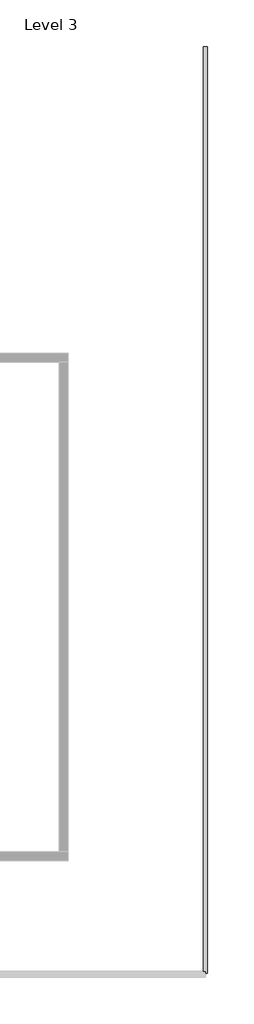
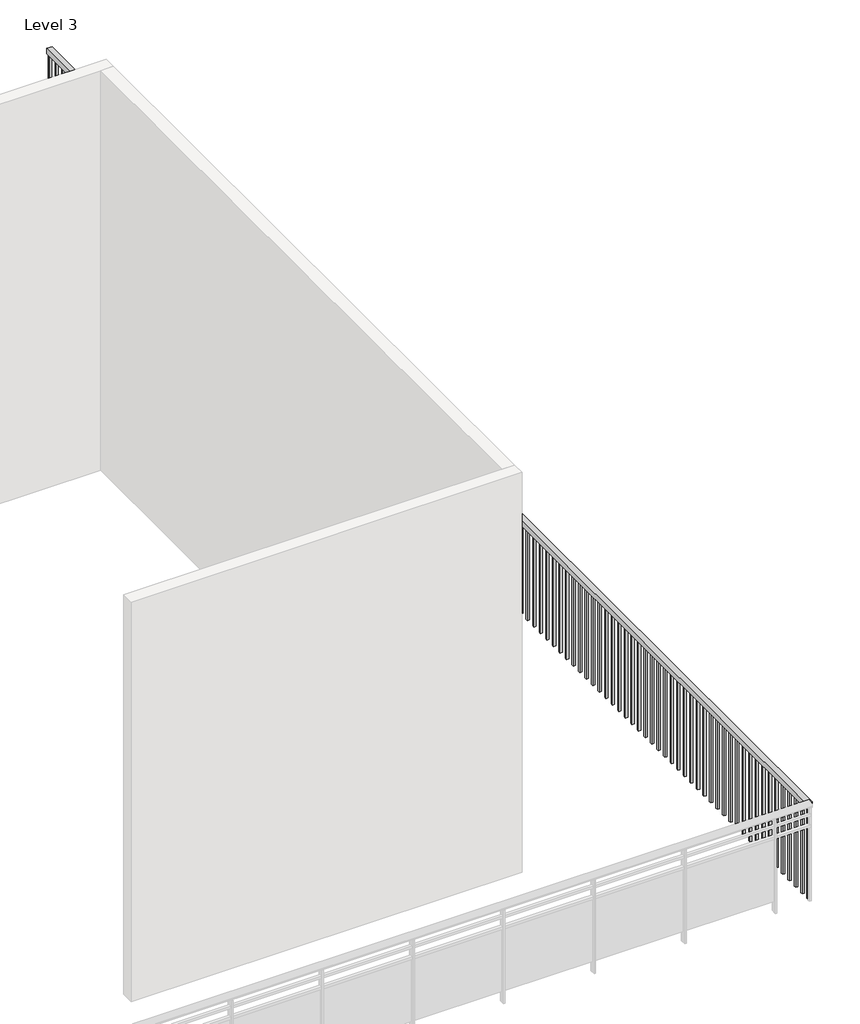
# One storey, part 2 of 2: 1 railing.
"""IFC4 building model written with IfcOpenShell, lengths in millimetres."""

from ifc_helpers import new_model, si_unit, frame, origin, place, context, project, spatial, polyline, outline, extrude, element, save

model = new_model("IFC4")

# Units and contexts
model_context = context("Model", 3, world=origin())
ifc_project = project(units=[si_unit("LENGTHUNIT", "METRE", prefix="MILLI")], contexts=[model_context])

# Site, building, storey
site = spatial("IfcSite", under=ifc_project)
building = spatial("IfcBuilding", under=site)
storey = spatial("IfcBuildingStorey", under=building, Name="Level 3", Elevation=3810.0)

# Railing
placement = place(None, origin())
element("IfcRailing", 1, ObjectType="Handrail - Rectangular", at=placement, inside=storey, context=model_context, shape_type="SweptSolid", body=[
    extrude(outline(polyline([(5557.6756121, -3130.6883122), (5506.8756121, -3130.6883122), (5506.8756121, 8667.6116878), (5557.6756121, 8667.6116878), (5557.6756121, -3130.6883122)])), frame((0.0, 0.0, 4673.6), z_axis=(0.0, 0.0, 1.0), x_axis=(1.0, 0.0, 0.0)), (0.0, 0.0, 1.0), 50.8),
    extrude(outline(polyline([(5541.8006121, 8645.3866878), (5522.7506121, 8645.3866878), (5522.7506121, 8664.4366878), (5541.8006121, 8664.4366878), (5541.8006121, 8645.3866878)])), frame((0.0, 0.0, 3810.0), z_axis=(0.0, 0.0, 1.0), x_axis=(1.0, 0.0, 0.0)), (0.0, 0.0, 1.0), 863.6),
    extrude(outline(polyline([(5541.8006121, 8543.7866878), (5522.7506121, 8543.7866878), (5522.7506121, 8562.8366878), (5541.8006121, 8562.8366878), (5541.8006121, 8543.7866878)])), frame((0.0, 0.0, 3810.0), z_axis=(0.0, 0.0, 1.0), x_axis=(1.0, 0.0, 0.0)), (0.0, 0.0, 1.0), 863.6),
    extrude(outline(polyline([(5541.8006121, 8442.1866878), (5522.7506121, 8442.1866878), (5522.7506121, 8461.2366878), (5541.8006121, 8461.2366878), (5541.8006121, 8442.1866878)])), frame((0.0, 0.0, 3810.0), z_axis=(0.0, 0.0, 1.0), x_axis=(1.0, 0.0, 0.0)), (0.0, 0.0, 1.0), 863.6),
    extrude(outline(polyline([(5541.8006121, 8340.5866878), (5522.7506121, 8340.5866878), (5522.7506121, 8359.6366878), (5541.8006121, 8359.6366878), (5541.8006121, 8340.5866878)])), frame((0.0, 0.0, 3810.0), z_axis=(0.0, 0.0, 1.0), x_axis=(1.0, 0.0, 0.0)), (0.0, 0.0, 1.0), 863.6),
    extrude(outline(polyline([(5541.8006121, 8238.9866878), (5522.7506121, 8238.9866878), (5522.7506121, 8258.0366878), (5541.8006121, 8258.0366878), (5541.8006121, 8238.9866878)])), frame((0.0, 0.0, 3810.0), z_axis=(0.0, 0.0, 1.0), x_axis=(1.0, 0.0, 0.0)), (0.0, 0.0, 1.0), 863.6),
    extrude(outline(polyline([(5541.8006121, 8137.3866878), (5522.7506121, 8137.3866878), (5522.7506121, 8156.4366878), (5541.8006121, 8156.4366878), (5541.8006121, 8137.3866878)])), frame((0.0, 0.0, 3810.0), z_axis=(0.0, 0.0, 1.0), x_axis=(1.0, 0.0, 0.0)), (0.0, 0.0, 1.0), 863.6),
    extrude(outline(polyline([(5541.8006121, 8035.7866878), (5522.7506121, 8035.7866878), (5522.7506121, 8054.8366878), (5541.8006121, 8054.8366878), (5541.8006121, 8035.7866878)])), frame((0.0, 0.0, 3810.0), z_axis=(0.0, 0.0, 1.0), x_axis=(1.0, 0.0, 0.0)), (0.0, 0.0, 1.0), 863.6),
    extrude(outline(polyline([(5541.8006121, 7934.1866878), (5522.7506121, 7934.1866878), (5522.7506121, 7953.2366878), (5541.8006121, 7953.2366878), (5541.8006121, 7934.1866878)])), frame((0.0, 0.0, 3810.0), z_axis=(0.0, 0.0, 1.0), x_axis=(1.0, 0.0, 0.0)), (0.0, 0.0, 1.0), 863.6),
    extrude(outline(polyline([(5541.8006121, 7832.5866878), (5522.7506121, 7832.5866878), (5522.7506121, 7851.6366878), (5541.8006121, 7851.6366878), (5541.8006121, 7832.5866878)])), frame((0.0, 0.0, 3810.0), z_axis=(0.0, 0.0, 1.0), x_axis=(1.0, 0.0, 0.0)), (0.0, 0.0, 1.0), 863.6),
    extrude(outline(polyline([(5541.8006121, 7730.9866878), (5522.7506121, 7730.9866878), (5522.7506121, 7750.0366878), (5541.8006121, 7750.0366878), (5541.8006121, 7730.9866878)])), frame((0.0, 0.0, 3810.0), z_axis=(0.0, 0.0, 1.0), x_axis=(1.0, 0.0, 0.0)), (0.0, 0.0, 1.0), 863.6),
    extrude(outline(polyline([(5541.8006121, 7629.3866878), (5522.7506121, 7629.3866878), (5522.7506121, 7648.4366878), (5541.8006121, 7648.4366878), (5541.8006121, 7629.3866878)])), frame((0.0, 0.0, 3810.0), z_axis=(0.0, 0.0, 1.0), x_axis=(1.0, 0.0, 0.0)), (0.0, 0.0, 1.0), 863.6),
    extrude(outline(polyline([(5541.8006121, 7527.7866878), (5522.7506121, 7527.7866878), (5522.7506121, 7546.8366878), (5541.8006121, 7546.8366878), (5541.8006121, 7527.7866878)])), frame((0.0, 0.0, 3810.0), z_axis=(0.0, 0.0, 1.0), x_axis=(1.0, 0.0, 0.0)), (0.0, 0.0, 1.0), 863.6),
    extrude(outline(polyline([(5541.8006121, 7426.1866878), (5522.7506121, 7426.1866878), (5522.7506121, 7445.2366878), (5541.8006121, 7445.2366878), (5541.8006121, 7426.1866878)])), frame((0.0, 0.0, 3810.0), z_axis=(0.0, 0.0, 1.0), x_axis=(1.0, 0.0, 0.0)), (0.0, 0.0, 1.0), 863.6),
    extrude(outline(polyline([(5541.8006121, 7324.5866878), (5522.7506121, 7324.5866878), (5522.7506121, 7343.6366878), (5541.8006121, 7343.6366878), (5541.8006121, 7324.5866878)])), frame((0.0, 0.0, 3810.0), z_axis=(0.0, 0.0, 1.0), x_axis=(1.0, 0.0, 0.0)), (0.0, 0.0, 1.0), 863.6),
    extrude(outline(polyline([(5541.8006121, 7222.9866878), (5522.7506121, 7222.9866878), (5522.7506121, 7242.0366878), (5541.8006121, 7242.0366878), (5541.8006121, 7222.9866878)])), frame((0.0, 0.0, 3810.0), z_axis=(0.0, 0.0, 1.0), x_axis=(1.0, 0.0, 0.0)), (0.0, 0.0, 1.0), 863.6),
    extrude(outline(polyline([(5541.8006121, 7121.3866878), (5522.7506121, 7121.3866878), (5522.7506121, 7140.4366878), (5541.8006121, 7140.4366878), (5541.8006121, 7121.3866878)])), frame((0.0, 0.0, 3810.0), z_axis=(0.0, 0.0, 1.0), x_axis=(1.0, 0.0, 0.0)), (0.0, 0.0, 1.0), 863.6),
    extrude(outline(polyline([(5541.8006121, 7019.7866878), (5522.7506121, 7019.7866878), (5522.7506121, 7038.8366878), (5541.8006121, 7038.8366878), (5541.8006121, 7019.7866878)])), frame((0.0, 0.0, 3810.0), z_axis=(0.0, 0.0, 1.0), x_axis=(1.0, 0.0, 0.0)), (0.0, 0.0, 1.0), 863.6),
    extrude(outline(polyline([(5541.8006121, 6918.1866878), (5522.7506121, 6918.1866878), (5522.7506121, 6937.2366878), (5541.8006121, 6937.2366878), (5541.8006121, 6918.1866878)])), frame((0.0, 0.0, 3810.0), z_axis=(0.0, 0.0, 1.0), x_axis=(1.0, 0.0, 0.0)), (0.0, 0.0, 1.0), 863.6),
    extrude(outline(polyline([(5541.8006121, 6816.5866878), (5522.7506121, 6816.5866878), (5522.7506121, 6835.6366878), (5541.8006121, 6835.6366878), (5541.8006121, 6816.5866878)])), frame((0.0, 0.0, 3810.0), z_axis=(0.0, 0.0, 1.0), x_axis=(1.0, 0.0, 0.0)), (0.0, 0.0, 1.0), 863.6),
    extrude(outline(polyline([(5541.8006121, 6714.9866878), (5522.7506121, 6714.9866878), (5522.7506121, 6734.0366878), (5541.8006121, 6734.0366878), (5541.8006121, 6714.9866878)])), frame((0.0, 0.0, 3810.0), z_axis=(0.0, 0.0, 1.0), x_axis=(1.0, 0.0, 0.0)), (0.0, 0.0, 1.0), 863.6),
    extrude(outline(polyline([(5541.8006121, 6613.3866878), (5522.7506121, 6613.3866878), (5522.7506121, 6632.4366878), (5541.8006121, 6632.4366878), (5541.8006121, 6613.3866878)])), frame((0.0, 0.0, 3810.0), z_axis=(0.0, 0.0, 1.0), x_axis=(1.0, 0.0, 0.0)), (0.0, 0.0, 1.0), 863.6),
    extrude(outline(polyline([(5541.8006121, 6511.7866878), (5522.7506121, 6511.7866878), (5522.7506121, 6530.8366878), (5541.8006121, 6530.8366878), (5541.8006121, 6511.7866878)])), frame((0.0, 0.0, 3810.0), z_axis=(0.0, 0.0, 1.0), x_axis=(1.0, 0.0, 0.0)), (0.0, 0.0, 1.0), 863.6),
    extrude(outline(polyline([(5541.8006121, 6410.1866878), (5522.7506121, 6410.1866878), (5522.7506121, 6429.2366878), (5541.8006121, 6429.2366878), (5541.8006121, 6410.1866878)])), frame((0.0, 0.0, 3810.0), z_axis=(0.0, 0.0, 1.0), x_axis=(1.0, 0.0, 0.0)), (0.0, 0.0, 1.0), 863.6),
    extrude(outline(polyline([(5541.8006121, 6308.5866878), (5522.7506121, 6308.5866878), (5522.7506121, 6327.6366878), (5541.8006121, 6327.6366878), (5541.8006121, 6308.5866878)])), frame((0.0, 0.0, 3810.0), z_axis=(0.0, 0.0, 1.0), x_axis=(1.0, 0.0, 0.0)), (0.0, 0.0, 1.0), 863.6),
    extrude(outline(polyline([(5541.8006121, 6206.9866878), (5522.7506121, 6206.9866878), (5522.7506121, 6226.0366878), (5541.8006121, 6226.0366878), (5541.8006121, 6206.9866878)])), frame((0.0, 0.0, 3810.0), z_axis=(0.0, 0.0, 1.0), x_axis=(1.0, 0.0, 0.0)), (0.0, 0.0, 1.0), 863.6),
    extrude(outline(polyline([(5541.8006121, 6105.3866878), (5522.7506121, 6105.3866878), (5522.7506121, 6124.4366878), (5541.8006121, 6124.4366878), (5541.8006121, 6105.3866878)])), frame((0.0, 0.0, 3810.0), z_axis=(0.0, 0.0, 1.0), x_axis=(1.0, 0.0, 0.0)), (0.0, 0.0, 1.0), 863.6),
    extrude(outline(polyline([(5541.8006121, 6003.7866878), (5522.7506121, 6003.7866878), (5522.7506121, 6022.8366878), (5541.8006121, 6022.8366878), (5541.8006121, 6003.7866878)])), frame((0.0, 0.0, 3810.0), z_axis=(0.0, 0.0, 1.0), x_axis=(1.0, 0.0, 0.0)), (0.0, 0.0, 1.0), 863.6),
    extrude(outline(polyline([(5541.8006121, 5902.1866878), (5522.7506121, 5902.1866878), (5522.7506121, 5921.2366878), (5541.8006121, 5921.2366878), (5541.8006121, 5902.1866878)])), frame((0.0, 0.0, 3810.0), z_axis=(0.0, 0.0, 1.0), x_axis=(1.0, 0.0, 0.0)), (0.0, 0.0, 1.0), 863.6),
    extrude(outline(polyline([(5541.8006121, 5800.5866878), (5522.7506121, 5800.5866878), (5522.7506121, 5819.6366878), (5541.8006121, 5819.6366878), (5541.8006121, 5800.5866878)])), frame((0.0, 0.0, 3810.0), z_axis=(0.0, 0.0, 1.0), x_axis=(1.0, 0.0, 0.0)), (0.0, 0.0, 1.0), 863.6),
    extrude(outline(polyline([(5541.8006121, 5698.9866878), (5522.7506121, 5698.9866878), (5522.7506121, 5718.0366878), (5541.8006121, 5718.0366878), (5541.8006121, 5698.9866878)])), frame((0.0, 0.0, 3810.0), z_axis=(0.0, 0.0, 1.0), x_axis=(1.0, 0.0, 0.0)), (0.0, 0.0, 1.0), 863.6),
    extrude(outline(polyline([(5541.8006121, 5597.3866878), (5522.7506121, 5597.3866878), (5522.7506121, 5616.4366878), (5541.8006121, 5616.4366878), (5541.8006121, 5597.3866878)])), frame((0.0, 0.0, 3810.0), z_axis=(0.0, 0.0, 1.0), x_axis=(1.0, 0.0, 0.0)), (0.0, 0.0, 1.0), 863.6),
    extrude(outline(polyline([(5541.8006121, 5495.7866878), (5522.7506121, 5495.7866878), (5522.7506121, 5514.8366878), (5541.8006121, 5514.8366878), (5541.8006121, 5495.7866878)])), frame((0.0, 0.0, 3810.0), z_axis=(0.0, 0.0, 1.0), x_axis=(1.0, 0.0, 0.0)), (0.0, 0.0, 1.0), 863.6),
    extrude(outline(polyline([(5541.8006121, 5394.1866878), (5522.7506121, 5394.1866878), (5522.7506121, 5413.2366878), (5541.8006121, 5413.2366878), (5541.8006121, 5394.1866878)])), frame((0.0, 0.0, 3810.0), z_axis=(0.0, 0.0, 1.0), x_axis=(1.0, 0.0, 0.0)), (0.0, 0.0, 1.0), 863.6),
    extrude(outline(polyline([(5541.8006121, 5292.5866878), (5522.7506121, 5292.5866878), (5522.7506121, 5311.6366878), (5541.8006121, 5311.6366878), (5541.8006121, 5292.5866878)])), frame((0.0, 0.0, 3810.0), z_axis=(0.0, 0.0, 1.0), x_axis=(1.0, 0.0, 0.0)), (0.0, 0.0, 1.0), 863.6),
    extrude(outline(polyline([(5541.8006121, 5190.9866878), (5522.7506121, 5190.9866878), (5522.7506121, 5210.0366878), (5541.8006121, 5210.0366878), (5541.8006121, 5190.9866878)])), frame((0.0, 0.0, 3810.0), z_axis=(0.0, 0.0, 1.0), x_axis=(1.0, 0.0, 0.0)), (0.0, 0.0, 1.0), 863.6),
    extrude(outline(polyline([(5541.8006121, 5089.3866878), (5522.7506121, 5089.3866878), (5522.7506121, 5108.4366878), (5541.8006121, 5108.4366878), (5541.8006121, 5089.3866878)])), frame((0.0, 0.0, 3810.0), z_axis=(0.0, 0.0, 1.0), x_axis=(1.0, 0.0, 0.0)), (0.0, 0.0, 1.0), 863.6),
    extrude(outline(polyline([(5541.8006121, 4987.7866878), (5522.7506121, 4987.7866878), (5522.7506121, 5006.8366878), (5541.8006121, 5006.8366878), (5541.8006121, 4987.7866878)])), frame((0.0, 0.0, 3810.0), z_axis=(0.0, 0.0, 1.0), x_axis=(1.0, 0.0, 0.0)), (0.0, 0.0, 1.0), 863.6),
    extrude(outline(polyline([(5541.8006121, 4886.1866878), (5522.7506121, 4886.1866878), (5522.7506121, 4905.2366878), (5541.8006121, 4905.2366878), (5541.8006121, 4886.1866878)])), frame((0.0, 0.0, 3810.0), z_axis=(0.0, 0.0, 1.0), x_axis=(1.0, 0.0, 0.0)), (0.0, 0.0, 1.0), 863.6),
    extrude(outline(polyline([(5541.8006121, 4784.5866878), (5522.7506121, 4784.5866878), (5522.7506121, 4803.6366878), (5541.8006121, 4803.6366878), (5541.8006121, 4784.5866878)])), frame((0.0, 0.0, 3810.0), z_axis=(0.0, 0.0, 1.0), x_axis=(1.0, 0.0, 0.0)), (0.0, 0.0, 1.0), 863.6),
    extrude(outline(polyline([(5541.8006121, 4682.9866878), (5522.7506121, 4682.9866878), (5522.7506121, 4702.0366878), (5541.8006121, 4702.0366878), (5541.8006121, 4682.9866878)])), frame((0.0, 0.0, 3810.0), z_axis=(0.0, 0.0, 1.0), x_axis=(1.0, 0.0, 0.0)), (0.0, 0.0, 1.0), 863.6),
    extrude(outline(polyline([(5541.8006121, 4581.3866878), (5522.7506121, 4581.3866878), (5522.7506121, 4600.4366878), (5541.8006121, 4600.4366878), (5541.8006121, 4581.3866878)])), frame((0.0, 0.0, 3810.0), z_axis=(0.0, 0.0, 1.0), x_axis=(1.0, 0.0, 0.0)), (0.0, 0.0, 1.0), 863.6),
    extrude(outline(polyline([(5541.8006121, 4479.7866878), (5522.7506121, 4479.7866878), (5522.7506121, 4498.8366878), (5541.8006121, 4498.8366878), (5541.8006121, 4479.7866878)])), frame((0.0, 0.0, 3810.0), z_axis=(0.0, 0.0, 1.0), x_axis=(1.0, 0.0, 0.0)), (0.0, 0.0, 1.0), 863.6),
    extrude(outline(polyline([(5541.8006121, 4378.1866878), (5522.7506121, 4378.1866878), (5522.7506121, 4397.2366878), (5541.8006121, 4397.2366878), (5541.8006121, 4378.1866878)])), frame((0.0, 0.0, 3810.0), z_axis=(0.0, 0.0, 1.0), x_axis=(1.0, 0.0, 0.0)), (0.0, 0.0, 1.0), 863.6),
    extrude(outline(polyline([(5541.8006121, 4276.5866878), (5522.7506121, 4276.5866878), (5522.7506121, 4295.6366878), (5541.8006121, 4295.6366878), (5541.8006121, 4276.5866878)])), frame((0.0, 0.0, 3810.0), z_axis=(0.0, 0.0, 1.0), x_axis=(1.0, 0.0, 0.0)), (0.0, 0.0, 1.0), 863.6),
    extrude(outline(polyline([(5541.8006121, 4174.9866878), (5522.7506121, 4174.9866878), (5522.7506121, 4194.0366878), (5541.8006121, 4194.0366878), (5541.8006121, 4174.9866878)])), frame((0.0, 0.0, 3810.0), z_axis=(0.0, 0.0, 1.0), x_axis=(1.0, 0.0, 0.0)), (0.0, 0.0, 1.0), 863.6),
    extrude(outline(polyline([(5541.8006121, 4073.3866878), (5522.7506121, 4073.3866878), (5522.7506121, 4092.4366878), (5541.8006121, 4092.4366878), (5541.8006121, 4073.3866878)])), frame((0.0, 0.0, 3810.0), z_axis=(0.0, 0.0, 1.0), x_axis=(1.0, 0.0, 0.0)), (0.0, 0.0, 1.0), 863.6),
    extrude(outline(polyline([(5541.8006121, 3971.7866878), (5522.7506121, 3971.7866878), (5522.7506121, 3990.8366878), (5541.8006121, 3990.8366878), (5541.8006121, 3971.7866878)])), frame((0.0, 0.0, 3810.0), z_axis=(0.0, 0.0, 1.0), x_axis=(1.0, 0.0, 0.0)), (0.0, 0.0, 1.0), 863.6),
    extrude(outline(polyline([(5541.8006121, 3870.1866878), (5522.7506121, 3870.1866878), (5522.7506121, 3889.2366878), (5541.8006121, 3889.2366878), (5541.8006121, 3870.1866878)])), frame((0.0, 0.0, 3810.0), z_axis=(0.0, 0.0, 1.0), x_axis=(1.0, 0.0, 0.0)), (0.0, 0.0, 1.0), 863.6),
    extrude(outline(polyline([(5541.8006121, 3768.5866878), (5522.7506121, 3768.5866878), (5522.7506121, 3787.6366878), (5541.8006121, 3787.6366878), (5541.8006121, 3768.5866878)])), frame((0.0, 0.0, 3810.0), z_axis=(0.0, 0.0, 1.0), x_axis=(1.0, 0.0, 0.0)), (0.0, 0.0, 1.0), 863.6),
    extrude(outline(polyline([(5541.8006121, 3666.9866878), (5522.7506121, 3666.9866878), (5522.7506121, 3686.0366878), (5541.8006121, 3686.0366878), (5541.8006121, 3666.9866878)])), frame((0.0, 0.0, 3810.0), z_axis=(0.0, 0.0, 1.0), x_axis=(1.0, 0.0, 0.0)), (0.0, 0.0, 1.0), 863.6),
    extrude(outline(polyline([(5541.8006121, 3565.3866878), (5522.7506121, 3565.3866878), (5522.7506121, 3584.4366878), (5541.8006121, 3584.4366878), (5541.8006121, 3565.3866878)])), frame((0.0, 0.0, 3810.0), z_axis=(0.0, 0.0, 1.0), x_axis=(1.0, 0.0, 0.0)), (0.0, 0.0, 1.0), 863.6),
    extrude(outline(polyline([(5541.8006121, 3463.7866878), (5522.7506121, 3463.7866878), (5522.7506121, 3482.8366878), (5541.8006121, 3482.8366878), (5541.8006121, 3463.7866878)])), frame((0.0, 0.0, 3810.0), z_axis=(0.0, 0.0, 1.0), x_axis=(1.0, 0.0, 0.0)), (0.0, 0.0, 1.0), 863.6),
    extrude(outline(polyline([(5541.8006121, 3362.1866878), (5522.7506121, 3362.1866878), (5522.7506121, 3381.2366878), (5541.8006121, 3381.2366878), (5541.8006121, 3362.1866878)])), frame((0.0, 0.0, 3810.0), z_axis=(0.0, 0.0, 1.0), x_axis=(1.0, 0.0, 0.0)), (0.0, 0.0, 1.0), 863.6),
    extrude(outline(polyline([(5541.8006121, 3260.5866878), (5522.7506121, 3260.5866878), (5522.7506121, 3279.6366878), (5541.8006121, 3279.6366878), (5541.8006121, 3260.5866878)])), frame((0.0, 0.0, 3810.0), z_axis=(0.0, 0.0, 1.0), x_axis=(1.0, 0.0, 0.0)), (0.0, 0.0, 1.0), 863.6),
    extrude(outline(polyline([(5541.8006121, 3158.9866878), (5522.7506121, 3158.9866878), (5522.7506121, 3178.0366878), (5541.8006121, 3178.0366878), (5541.8006121, 3158.9866878)])), frame((0.0, 0.0, 3810.0), z_axis=(0.0, 0.0, 1.0), x_axis=(1.0, 0.0, 0.0)), (0.0, 0.0, 1.0), 863.6),
    extrude(outline(polyline([(5541.8006121, 3057.3866878), (5522.7506121, 3057.3866878), (5522.7506121, 3076.4366878), (5541.8006121, 3076.4366878), (5541.8006121, 3057.3866878)])), frame((0.0, 0.0, 3810.0), z_axis=(0.0, 0.0, 1.0), x_axis=(1.0, 0.0, 0.0)), (0.0, 0.0, 1.0), 863.6),
    extrude(outline(polyline([(5541.8006121, 2955.7866878), (5522.7506121, 2955.7866878), (5522.7506121, 2974.8366878), (5541.8006121, 2974.8366878), (5541.8006121, 2955.7866878)])), frame((0.0, 0.0, 3810.0), z_axis=(0.0, 0.0, 1.0), x_axis=(1.0, 0.0, 0.0)), (0.0, 0.0, 1.0), 863.6),
    extrude(outline(polyline([(5541.8006121, 2854.1866878), (5522.7506121, 2854.1866878), (5522.7506121, 2873.2366878), (5541.8006121, 2873.2366878), (5541.8006121, 2854.1866878)])), frame((0.0, 0.0, 3810.0), z_axis=(0.0, 0.0, 1.0), x_axis=(1.0, 0.0, 0.0)), (0.0, 0.0, 1.0), 863.6),
    extrude(outline(polyline([(5541.8006121, 2752.5866878), (5522.7506121, 2752.5866878), (5522.7506121, 2771.6366878), (5541.8006121, 2771.6366878), (5541.8006121, 2752.5866878)])), frame((0.0, 0.0, 3810.0), z_axis=(0.0, 0.0, 1.0), x_axis=(1.0, 0.0, 0.0)), (0.0, 0.0, 1.0), 863.6),
    extrude(outline(polyline([(5541.8006121, 2650.9866878), (5522.7506121, 2650.9866878), (5522.7506121, 2670.0366878), (5541.8006121, 2670.0366878), (5541.8006121, 2650.9866878)])), frame((0.0, 0.0, 3810.0), z_axis=(0.0, 0.0, 1.0), x_axis=(1.0, 0.0, 0.0)), (0.0, 0.0, 1.0), 863.6),
    extrude(outline(polyline([(5541.8006121, 2549.3866878), (5522.7506121, 2549.3866878), (5522.7506121, 2568.4366878), (5541.8006121, 2568.4366878), (5541.8006121, 2549.3866878)])), frame((0.0, 0.0, 3810.0), z_axis=(0.0, 0.0, 1.0), x_axis=(1.0, 0.0, 0.0)), (0.0, 0.0, 1.0), 863.6),
    extrude(outline(polyline([(5541.8006121, 2447.7866878), (5522.7506121, 2447.7866878), (5522.7506121, 2466.8366878), (5541.8006121, 2466.8366878), (5541.8006121, 2447.7866878)])), frame((0.0, 0.0, 3810.0), z_axis=(0.0, 0.0, 1.0), x_axis=(1.0, 0.0, 0.0)), (0.0, 0.0, 1.0), 863.6),
    extrude(outline(polyline([(5541.8006121, 2346.1866878), (5522.7506121, 2346.1866878), (5522.7506121, 2365.2366878), (5541.8006121, 2365.2366878), (5541.8006121, 2346.1866878)])), frame((0.0, 0.0, 3810.0), z_axis=(0.0, 0.0, 1.0), x_axis=(1.0, 0.0, 0.0)), (0.0, 0.0, 1.0), 863.6),
    extrude(outline(polyline([(5541.8006121, 2244.5866878), (5522.7506121, 2244.5866878), (5522.7506121, 2263.6366878), (5541.8006121, 2263.6366878), (5541.8006121, 2244.5866878)])), frame((0.0, 0.0, 3810.0), z_axis=(0.0, 0.0, 1.0), x_axis=(1.0, 0.0, 0.0)), (0.0, 0.0, 1.0), 863.6),
    extrude(outline(polyline([(5541.8006121, 2142.9866878), (5522.7506121, 2142.9866878), (5522.7506121, 2162.0366878), (5541.8006121, 2162.0366878), (5541.8006121, 2142.9866878)])), frame((0.0, 0.0, 3810.0), z_axis=(0.0, 0.0, 1.0), x_axis=(1.0, 0.0, 0.0)), (0.0, 0.0, 1.0), 863.6),
    extrude(outline(polyline([(5541.8006121, 2041.3866878), (5522.7506121, 2041.3866878), (5522.7506121, 2060.4366878), (5541.8006121, 2060.4366878), (5541.8006121, 2041.3866878)])), frame((0.0, 0.0, 3810.0), z_axis=(0.0, 0.0, 1.0), x_axis=(1.0, 0.0, 0.0)), (0.0, 0.0, 1.0), 863.6),
    extrude(outline(polyline([(5541.8006121, 1939.7866878), (5522.7506121, 1939.7866878), (5522.7506121, 1958.8366878), (5541.8006121, 1958.8366878), (5541.8006121, 1939.7866878)])), frame((0.0, 0.0, 3810.0), z_axis=(0.0, 0.0, 1.0), x_axis=(1.0, 0.0, 0.0)), (0.0, 0.0, 1.0), 863.6),
    extrude(outline(polyline([(5541.8006121, 1838.1866878), (5522.7506121, 1838.1866878), (5522.7506121, 1857.2366878), (5541.8006121, 1857.2366878), (5541.8006121, 1838.1866878)])), frame((0.0, 0.0, 3810.0), z_axis=(0.0, 0.0, 1.0), x_axis=(1.0, 0.0, 0.0)), (0.0, 0.0, 1.0), 863.6),
    extrude(outline(polyline([(5541.8006121, 1736.5866878), (5522.7506121, 1736.5866878), (5522.7506121, 1755.6366878), (5541.8006121, 1755.6366878), (5541.8006121, 1736.5866878)])), frame((0.0, 0.0, 3810.0), z_axis=(0.0, 0.0, 1.0), x_axis=(1.0, 0.0, 0.0)), (0.0, 0.0, 1.0), 863.6),
    extrude(outline(polyline([(5541.8006121, 1634.9866878), (5522.7506121, 1634.9866878), (5522.7506121, 1654.0366878), (5541.8006121, 1654.0366878), (5541.8006121, 1634.9866878)])), frame((0.0, 0.0, 3810.0), z_axis=(0.0, 0.0, 1.0), x_axis=(1.0, 0.0, 0.0)), (0.0, 0.0, 1.0), 863.6),
    extrude(outline(polyline([(5541.8006121, 1533.3866878), (5522.7506121, 1533.3866878), (5522.7506121, 1552.4366878), (5541.8006121, 1552.4366878), (5541.8006121, 1533.3866878)])), frame((0.0, 0.0, 3810.0), z_axis=(0.0, 0.0, 1.0), x_axis=(1.0, 0.0, 0.0)), (0.0, 0.0, 1.0), 863.6),
    extrude(outline(polyline([(5541.8006121, 1431.7866878), (5522.7506121, 1431.7866878), (5522.7506121, 1450.8366878), (5541.8006121, 1450.8366878), (5541.8006121, 1431.7866878)])), frame((0.0, 0.0, 3810.0), z_axis=(0.0, 0.0, 1.0), x_axis=(1.0, 0.0, 0.0)), (0.0, 0.0, 1.0), 863.6),
    extrude(outline(polyline([(5541.8006121, 1330.1866878), (5522.7506121, 1330.1866878), (5522.7506121, 1349.2366878), (5541.8006121, 1349.2366878), (5541.8006121, 1330.1866878)])), frame((0.0, 0.0, 3810.0), z_axis=(0.0, 0.0, 1.0), x_axis=(1.0, 0.0, 0.0)), (0.0, 0.0, 1.0), 863.6),
    extrude(outline(polyline([(5541.8006121, 1228.5866878), (5522.7506121, 1228.5866878), (5522.7506121, 1247.6366878), (5541.8006121, 1247.6366878), (5541.8006121, 1228.5866878)])), frame((0.0, 0.0, 3810.0), z_axis=(0.0, 0.0, 1.0), x_axis=(1.0, 0.0, 0.0)), (0.0, 0.0, 1.0), 863.6),
    extrude(outline(polyline([(5541.8006121, 1126.9866878), (5522.7506121, 1126.9866878), (5522.7506121, 1146.0366878), (5541.8006121, 1146.0366878), (5541.8006121, 1126.9866878)])), frame((0.0, 0.0, 3810.0), z_axis=(0.0, 0.0, 1.0), x_axis=(1.0, 0.0, 0.0)), (0.0, 0.0, 1.0), 863.6),
    extrude(outline(polyline([(5541.8006121, 1025.3866878), (5522.7506121, 1025.3866878), (5522.7506121, 1044.4366878), (5541.8006121, 1044.4366878), (5541.8006121, 1025.3866878)])), frame((0.0, 0.0, 3810.0), z_axis=(0.0, 0.0, 1.0), x_axis=(1.0, 0.0, 0.0)), (0.0, 0.0, 1.0), 863.6),
    extrude(outline(polyline([(5541.8006121, 923.7866878), (5522.7506121, 923.7866878), (5522.7506121, 942.8366878), (5541.8006121, 942.8366878), (5541.8006121, 923.7866878)])), frame((0.0, 0.0, 3810.0), z_axis=(0.0, 0.0, 1.0), x_axis=(1.0, 0.0, 0.0)), (0.0, 0.0, 1.0), 863.6),
    extrude(outline(polyline([(5541.8006121, 822.1866878), (5522.7506121, 822.1866878), (5522.7506121, 841.2366878), (5541.8006121, 841.2366878), (5541.8006121, 822.1866878)])), frame((0.0, 0.0, 3810.0), z_axis=(0.0, 0.0, 1.0), x_axis=(1.0, 0.0, 0.0)), (0.0, 0.0, 1.0), 863.6),
    extrude(outline(polyline([(5541.8006121, 720.5866878), (5522.7506121, 720.5866878), (5522.7506121, 739.6366878), (5541.8006121, 739.6366878), (5541.8006121, 720.5866878)])), frame((0.0, 0.0, 3810.0), z_axis=(0.0, 0.0, 1.0), x_axis=(1.0, 0.0, 0.0)), (0.0, 0.0, 1.0), 863.6),
    extrude(outline(polyline([(5541.8006121, 618.9866878), (5522.7506121, 618.9866878), (5522.7506121, 638.0366878), (5541.8006121, 638.0366878), (5541.8006121, 618.9866878)])), frame((0.0, 0.0, 3810.0), z_axis=(0.0, 0.0, 1.0), x_axis=(1.0, 0.0, 0.0)), (0.0, 0.0, 1.0), 863.6),
    extrude(outline(polyline([(5541.8006121, 517.3866878), (5522.7506121, 517.3866878), (5522.7506121, 536.4366878), (5541.8006121, 536.4366878), (5541.8006121, 517.3866878)])), frame((0.0, 0.0, 3810.0), z_axis=(0.0, 0.0, 1.0), x_axis=(1.0, 0.0, 0.0)), (0.0, 0.0, 1.0), 863.6),
    extrude(outline(polyline([(5541.8006121, 415.7866878), (5522.7506121, 415.7866878), (5522.7506121, 434.8366878), (5541.8006121, 434.8366878), (5541.8006121, 415.7866878)])), frame((0.0, 0.0, 3810.0), z_axis=(0.0, 0.0, 1.0), x_axis=(1.0, 0.0, 0.0)), (0.0, 0.0, 1.0), 863.6),
    extrude(outline(polyline([(5541.8006121, 314.1866878), (5522.7506121, 314.1866878), (5522.7506121, 333.2366878), (5541.8006121, 333.2366878), (5541.8006121, 314.1866878)])), frame((0.0, 0.0, 3810.0), z_axis=(0.0, 0.0, 1.0), x_axis=(1.0, 0.0, 0.0)), (0.0, 0.0, 1.0), 863.6),
    extrude(outline(polyline([(5541.8006121, 212.5866878), (5522.7506121, 212.5866878), (5522.7506121, 231.6366878), (5541.8006121, 231.6366878), (5541.8006121, 212.5866878)])), frame((0.0, 0.0, 3810.0), z_axis=(0.0, 0.0, 1.0), x_axis=(1.0, 0.0, 0.0)), (0.0, 0.0, 1.0), 863.6),
    extrude(outline(polyline([(5541.8006121, 110.9866878), (5522.7506121, 110.9866878), (5522.7506121, 130.0366878), (5541.8006121, 130.0366878), (5541.8006121, 110.9866878)])), frame((0.0, 0.0, 3810.0), z_axis=(0.0, 0.0, 1.0), x_axis=(1.0, 0.0, 0.0)), (0.0, 0.0, 1.0), 863.6),
    extrude(outline(polyline([(5541.8006121, 9.3866878), (5522.7506121, 9.3866878), (5522.7506121, 28.4366878), (5541.8006121, 28.4366878), (5541.8006121, 9.3866878)])), frame((0.0, 0.0, 3810.0), z_axis=(0.0, 0.0, 1.0), x_axis=(1.0, 0.0, 0.0)), (0.0, 0.0, 1.0), 863.6),
    extrude(outline(polyline([(5541.8006121, -92.2133122), (5522.7506121, -92.2133122), (5522.7506121, -73.1633122), (5541.8006121, -73.1633122), (5541.8006121, -92.2133122)])), frame((0.0, 0.0, 3810.0), z_axis=(0.0, 0.0, 1.0), x_axis=(1.0, 0.0, 0.0)), (0.0, 0.0, 1.0), 863.6),
    extrude(outline(polyline([(5541.8006121, -193.8133122), (5522.7506121, -193.8133122), (5522.7506121, -174.7633122), (5541.8006121, -174.7633122), (5541.8006121, -193.8133122)])), frame((0.0, 0.0, 3810.0), z_axis=(0.0, 0.0, 1.0), x_axis=(1.0, 0.0, 0.0)), (0.0, 0.0, 1.0), 863.6),
    extrude(outline(polyline([(5541.8006121, -295.4133122), (5522.7506121, -295.4133122), (5522.7506121, -276.3633122), (5541.8006121, -276.3633122), (5541.8006121, -295.4133122)])), frame((0.0, 0.0, 3810.0), z_axis=(0.0, 0.0, 1.0), x_axis=(1.0, 0.0, 0.0)), (0.0, 0.0, 1.0), 863.6),
    extrude(outline(polyline([(5541.8006121, -397.0133122), (5522.7506121, -397.0133122), (5522.7506121, -377.9633122), (5541.8006121, -377.9633122), (5541.8006121, -397.0133122)])), frame((0.0, 0.0, 3810.0), z_axis=(0.0, 0.0, 1.0), x_axis=(1.0, 0.0, 0.0)), (0.0, 0.0, 1.0), 863.6),
    extrude(outline(polyline([(5541.8006121, -498.6133122), (5522.7506121, -498.6133122), (5522.7506121, -479.5633122), (5541.8006121, -479.5633122), (5541.8006121, -498.6133122)])), frame((0.0, 0.0, 3810.0), z_axis=(0.0, 0.0, 1.0), x_axis=(1.0, 0.0, 0.0)), (0.0, 0.0, 1.0), 863.6),
    extrude(outline(polyline([(5541.8006121, -600.2133122), (5522.7506121, -600.2133122), (5522.7506121, -581.1633122), (5541.8006121, -581.1633122), (5541.8006121, -600.2133122)])), frame((0.0, 0.0, 3810.0), z_axis=(0.0, 0.0, 1.0), x_axis=(1.0, 0.0, 0.0)), (0.0, 0.0, 1.0), 863.6),
    extrude(outline(polyline([(5541.8006121, -701.8133122), (5522.7506121, -701.8133122), (5522.7506121, -682.7633122), (5541.8006121, -682.7633122), (5541.8006121, -701.8133122)])), frame((0.0, 0.0, 3810.0), z_axis=(0.0, 0.0, 1.0), x_axis=(1.0, 0.0, 0.0)), (0.0, 0.0, 1.0), 863.6),
    extrude(outline(polyline([(5541.8006121, -803.4133122), (5522.7506121, -803.4133122), (5522.7506121, -784.3633122), (5541.8006121, -784.3633122), (5541.8006121, -803.4133122)])), frame((0.0, 0.0, 3810.0), z_axis=(0.0, 0.0, 1.0), x_axis=(1.0, 0.0, 0.0)), (0.0, 0.0, 1.0), 863.6),
    extrude(outline(polyline([(5541.8006121, -905.0133122), (5522.7506121, -905.0133122), (5522.7506121, -885.9633122), (5541.8006121, -885.9633122), (5541.8006121, -905.0133122)])), frame((0.0, 0.0, 3810.0), z_axis=(0.0, 0.0, 1.0), x_axis=(1.0, 0.0, 0.0)), (0.0, 0.0, 1.0), 863.6),
    extrude(outline(polyline([(5541.8006121, -1006.6133122), (5522.7506121, -1006.6133122), (5522.7506121, -987.5633122), (5541.8006121, -987.5633122), (5541.8006121, -1006.6133122)])), frame((0.0, 0.0, 3810.0), z_axis=(0.0, 0.0, 1.0), x_axis=(1.0, 0.0, 0.0)), (0.0, 0.0, 1.0), 863.6),
    extrude(outline(polyline([(5541.8006121, -1108.2133122), (5522.7506121, -1108.2133122), (5522.7506121, -1089.1633122), (5541.8006121, -1089.1633122), (5541.8006121, -1108.2133122)])), frame((0.0, 0.0, 3810.0), z_axis=(0.0, 0.0, 1.0), x_axis=(1.0, 0.0, 0.0)), (0.0, 0.0, 1.0), 863.6),
    extrude(outline(polyline([(5541.8006121, -1209.8133122), (5522.7506121, -1209.8133122), (5522.7506121, -1190.7633122), (5541.8006121, -1190.7633122), (5541.8006121, -1209.8133122)])), frame((0.0, 0.0, 3810.0), z_axis=(0.0, 0.0, 1.0), x_axis=(1.0, 0.0, 0.0)), (0.0, 0.0, 1.0), 863.6),
    extrude(outline(polyline([(5541.8006121, -1311.4133122), (5522.7506121, -1311.4133122), (5522.7506121, -1292.3633122), (5541.8006121, -1292.3633122), (5541.8006121, -1311.4133122)])), frame((0.0, 0.0, 3810.0), z_axis=(0.0, 0.0, 1.0), x_axis=(1.0, 0.0, 0.0)), (0.0, 0.0, 1.0), 863.6),
    extrude(outline(polyline([(5541.8006121, -1413.0133122), (5522.7506121, -1413.0133122), (5522.7506121, -1393.9633122), (5541.8006121, -1393.9633122), (5541.8006121, -1413.0133122)])), frame((0.0, 0.0, 3810.0), z_axis=(0.0, 0.0, 1.0), x_axis=(1.0, 0.0, 0.0)), (0.0, 0.0, 1.0), 863.6),
    extrude(outline(polyline([(5541.8006121, -1514.6133122), (5522.7506121, -1514.6133122), (5522.7506121, -1495.5633122), (5541.8006121, -1495.5633122), (5541.8006121, -1514.6133122)])), frame((0.0, 0.0, 3810.0), z_axis=(0.0, 0.0, 1.0), x_axis=(1.0, 0.0, 0.0)), (0.0, 0.0, 1.0), 863.6),
    extrude(outline(polyline([(5541.8006121, -1616.2133122), (5522.7506121, -1616.2133122), (5522.7506121, -1597.1633122), (5541.8006121, -1597.1633122), (5541.8006121, -1616.2133122)])), frame((0.0, 0.0, 3810.0), z_axis=(0.0, 0.0, 1.0), x_axis=(1.0, 0.0, 0.0)), (0.0, 0.0, 1.0), 863.6),
    extrude(outline(polyline([(5541.8006121, -1717.8133122), (5522.7506121, -1717.8133122), (5522.7506121, -1698.7633122), (5541.8006121, -1698.7633122), (5541.8006121, -1717.8133122)])), frame((0.0, 0.0, 3810.0), z_axis=(0.0, 0.0, 1.0), x_axis=(1.0, 0.0, 0.0)), (0.0, 0.0, 1.0), 863.6),
    extrude(outline(polyline([(5541.8006121, -1819.4133122), (5522.7506121, -1819.4133122), (5522.7506121, -1800.3633122), (5541.8006121, -1800.3633122), (5541.8006121, -1819.4133122)])), frame((0.0, 0.0, 3810.0), z_axis=(0.0, 0.0, 1.0), x_axis=(1.0, 0.0, 0.0)), (0.0, 0.0, 1.0), 863.6),
    extrude(outline(polyline([(5541.8006121, -1921.0133122), (5522.7506121, -1921.0133122), (5522.7506121, -1901.9633122), (5541.8006121, -1901.9633122), (5541.8006121, -1921.0133122)])), frame((0.0, 0.0, 3810.0), z_axis=(0.0, 0.0, 1.0), x_axis=(1.0, 0.0, 0.0)), (0.0, 0.0, 1.0), 863.6),
    extrude(outline(polyline([(5541.8006121, -2022.6133122), (5522.7506121, -2022.6133122), (5522.7506121, -2003.5633122), (5541.8006121, -2003.5633122), (5541.8006121, -2022.6133122)])), frame((0.0, 0.0, 3810.0), z_axis=(0.0, 0.0, 1.0), x_axis=(1.0, 0.0, 0.0)), (0.0, 0.0, 1.0), 863.6),
    extrude(outline(polyline([(5541.8006121, -2124.2133122), (5522.7506121, -2124.2133122), (5522.7506121, -2105.1633122), (5541.8006121, -2105.1633122), (5541.8006121, -2124.2133122)])), frame((0.0, 0.0, 3810.0), z_axis=(0.0, 0.0, 1.0), x_axis=(1.0, 0.0, 0.0)), (0.0, 0.0, 1.0), 863.6),
    extrude(outline(polyline([(5541.8006121, -2225.8133122), (5522.7506121, -2225.8133122), (5522.7506121, -2206.7633122), (5541.8006121, -2206.7633122), (5541.8006121, -2225.8133122)])), frame((0.0, 0.0, 3810.0), z_axis=(0.0, 0.0, 1.0), x_axis=(1.0, 0.0, 0.0)), (0.0, 0.0, 1.0), 863.6),
    extrude(outline(polyline([(5541.8006121, -2327.4133122), (5522.7506121, -2327.4133122), (5522.7506121, -2308.3633122), (5541.8006121, -2308.3633122), (5541.8006121, -2327.4133122)])), frame((0.0, 0.0, 3810.0), z_axis=(0.0, 0.0, 1.0), x_axis=(1.0, 0.0, 0.0)), (0.0, 0.0, 1.0), 863.6),
    extrude(outline(polyline([(5541.8006121, -2429.0133122), (5522.7506121, -2429.0133122), (5522.7506121, -2409.9633122), (5541.8006121, -2409.9633122), (5541.8006121, -2429.0133122)])), frame((0.0, 0.0, 3810.0), z_axis=(0.0, 0.0, 1.0), x_axis=(1.0, 0.0, 0.0)), (0.0, 0.0, 1.0), 863.6),
    extrude(outline(polyline([(5541.8006121, -2530.6133122), (5522.7506121, -2530.6133122), (5522.7506121, -2511.5633122), (5541.8006121, -2511.5633122), (5541.8006121, -2530.6133122)])), frame((0.0, 0.0, 3810.0), z_axis=(0.0, 0.0, 1.0), x_axis=(1.0, 0.0, 0.0)), (0.0, 0.0, 1.0), 863.6),
    extrude(outline(polyline([(5541.8006121, -2632.2133122), (5522.7506121, -2632.2133122), (5522.7506121, -2613.1633122), (5541.8006121, -2613.1633122), (5541.8006121, -2632.2133122)])), frame((0.0, 0.0, 3810.0), z_axis=(0.0, 0.0, 1.0), x_axis=(1.0, 0.0, 0.0)), (0.0, 0.0, 1.0), 863.6),
    extrude(outline(polyline([(5541.8006121, -2733.8133122), (5522.7506121, -2733.8133122), (5522.7506121, -2714.7633122), (5541.8006121, -2714.7633122), (5541.8006121, -2733.8133122)])), frame((0.0, 0.0, 3810.0), z_axis=(0.0, 0.0, 1.0), x_axis=(1.0, 0.0, 0.0)), (0.0, 0.0, 1.0), 863.6),
    extrude(outline(polyline([(5541.8006121, -2835.4133122), (5522.7506121, -2835.4133122), (5522.7506121, -2816.3633122), (5541.8006121, -2816.3633122), (5541.8006121, -2835.4133122)])), frame((0.0, 0.0, 3810.0), z_axis=(0.0, 0.0, 1.0), x_axis=(1.0, 0.0, 0.0)), (0.0, 0.0, 1.0), 863.6),
    extrude(outline(polyline([(5541.8006121, -2937.0133122), (5522.7506121, -2937.0133122), (5522.7506121, -2917.9633122), (5541.8006121, -2917.9633122), (5541.8006121, -2937.0133122)])), frame((0.0, 0.0, 3810.0), z_axis=(0.0, 0.0, 1.0), x_axis=(1.0, 0.0, 0.0)), (0.0, 0.0, 1.0), 863.6),
    extrude(outline(polyline([(5541.8006121, -3038.6133122), (5522.7506121, -3038.6133122), (5522.7506121, -3019.5633122), (5541.8006121, -3019.5633122), (5541.8006121, -3038.6133122)])), frame((0.0, 0.0, 3810.0), z_axis=(0.0, 0.0, 1.0), x_axis=(1.0, 0.0, 0.0)), (0.0, 0.0, 1.0), 863.6),
    extrude(outline(polyline([(5541.8006121, 8648.5616878), (5522.7506121, 8648.5616878), (5522.7506121, 8667.6116878), (5541.8006121, 8667.6116878), (5541.8006121, 8648.5616878)])), frame((0.0, 0.0, 3810.0), z_axis=(0.0, 0.0, 1.0), x_axis=(1.0, 0.0, 0.0)), (0.0, 0.0, 1.0), 863.6),
    extrude(outline(polyline([(5541.8006121, -3130.6883122), (5522.7506121, -3130.6883122), (5522.7506121, -3111.6383122), (5541.8006121, -3111.6383122), (5541.8006121, -3130.6883122)])), frame((0.0, 0.0, 3810.0), z_axis=(0.0, 0.0, 1.0), x_axis=(1.0, 0.0, 0.0)), (0.0, 0.0, 1.0), 863.6),
])

save(model, "model.ifc")

# Revit data of these elements
# Type "Handrail - Rectangular"
#   Assembly Code = "C2010400"
#   built-in parameter 1008612 = 0.0416667 (stored number, unit not read)
#   built-in parameter 1008611 = 0.0416667 (stored number, unit not read)
#   built-in parameter 1008609 = 0.333333 (stored number, unit not read)
#   built-in parameter 1008604 = 0.166667 (stored number, unit not read)
#   built-in parameter 1008603 = 0.166667 (stored number, unit not read)
#   Railing Height = 3' - 0"
#   built-in parameter 1008630 = 2
#   built-in parameter 1008610 = 2
#   built-in parameter 1008618 = Baluster - Square : 3/4"
# Element 1 (IfcRailing, "Handrail - Rectangular")
#   Phase Created = New Construction
